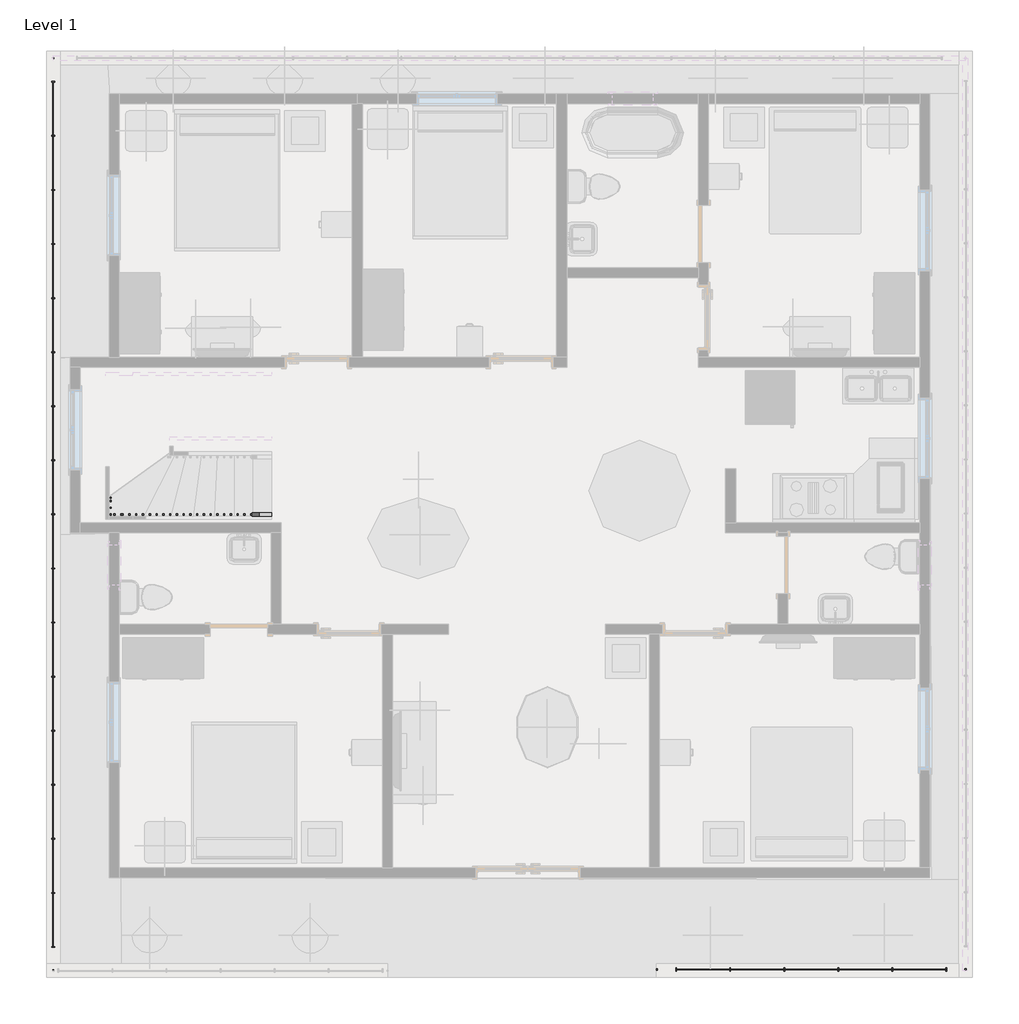
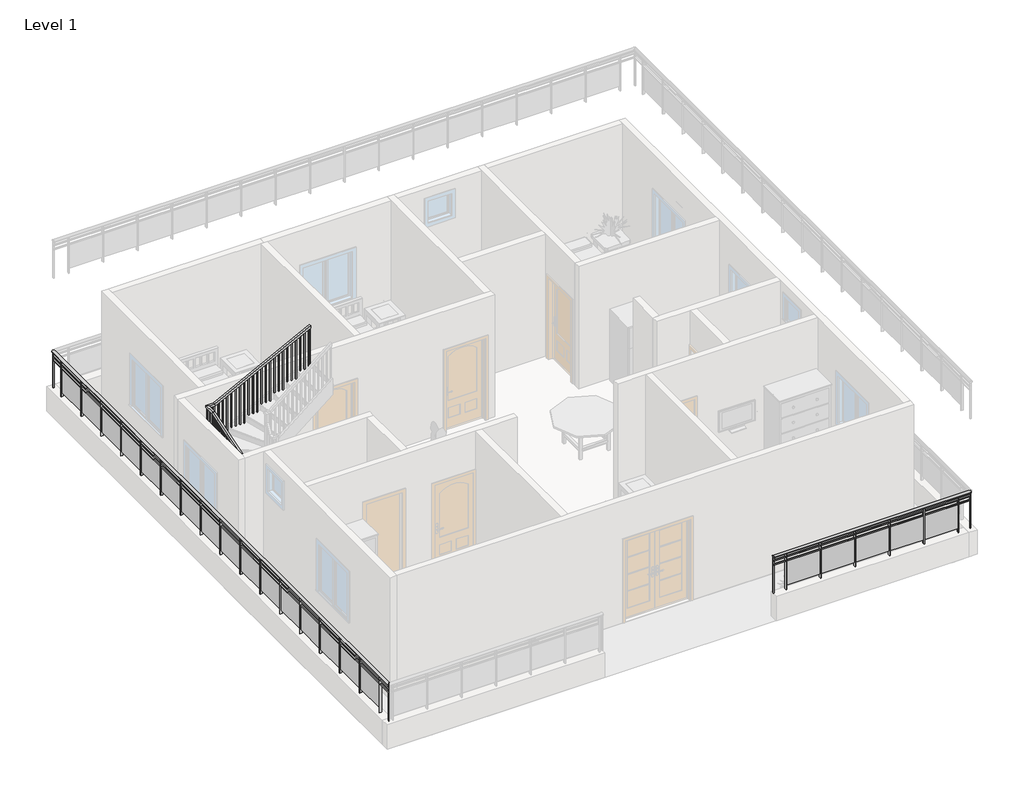
# One storey, part 2 of 5: 3 railings.
"""IFC4 building model written with IfcOpenShell, lengths in millimetres."""

from ifc_helpers import new_model, si_unit, point, frame, origin, place, context, project, spatial, polyline, ellipse_curve, trimmed, outline, extrude, faceted_brep, element, save
from ifc_brep_helpers import plane_surface, extruded_surface, advanced_brep

model = new_model("IFC4")

# Units and contexts
model_context = context("Model", 3, world=origin())
ifc_project = project(units=[si_unit("LENGTHUNIT", "METRE", prefix="MILLI")], contexts=[model_context])

# Site, building, storey
site = spatial("IfcSite", under=ifc_project)
building = spatial("IfcBuilding", under=site)
storey = spatial("IfcBuildingStorey", under=building, Name="Level 1", Elevation=0.0)

# Railings
placement = place(None, origin())
element("IfcRailing", 1, ObjectType="Glass Panel - Bottom Fill", at=placement, inside=storey, context=model_context, shape_type="SolidModel", body=[
    advanced_brep(
    [(2243.3065334, 607.1216937, 1524.0), (2243.3065334, 683.3216937, 1524.0), (-2404.8934666, 607.1216937, 1524.0), (-2404.8934666, 683.3216937, 1524.0)],
    [
        (0, 1, ellipse_curve(frame((2243.3065334, 645.2216937, 1524.0), z_axis=(1.0, 0.0, 0.0), x_axis=(0.0, 1.0, 0.0)), 38.1, 28.575)),
        (1, 0, ellipse_curve(frame((2243.3065334, 645.2216937, 1524.0), z_axis=(1.0, 0.0, 0.0), x_axis=(0.0, 1.0, 0.0)), 38.1, 28.575)),
        (2, 3, ellipse_curve(frame((-2404.8934666, 645.2216937, 1524.0), z_axis=(-1.0, 0.0, 0.0), x_axis=(0.0, 1.0, 0.0)), 38.1, 28.575)),
        (3, 2, ellipse_curve(frame((-2404.8934666, 645.2216937, 1524.0), z_axis=(-1.0, 0.0, 0.0), x_axis=(0.0, 1.0, 0.0)), 38.1, 28.575)),
        (0, 2),
        (3, 1),
    ],
    [
        plane_surface(frame((2243.3065334, 645.2216937, 1524.0), z_axis=(1.0, 0.0, 0.0), x_axis=(0.0, -1.0, 0.0))),
        plane_surface(frame((-2404.8934666, 645.2216937, 1524.0), z_axis=(-1.0, 0.0, 0.0), x_axis=(0.0, -1.0, 0.0))),
        extruded_surface(trimmed(ellipse_curve(frame((-2404.8934666, 645.2216937, 1524.0), z_axis=(1.0, 0.0, 0.0), x_axis=(0.0, 1.0, 0.0)), 38.1, 28.575), [point((-2404.8934666, 607.1216937, 1524.0))], [point((-2404.8934666, 683.3216937, 1524.0))], True, "CARTESIAN"), (4648.2, 0.0, 0.0), 4648.2),
        extruded_surface(trimmed(ellipse_curve(frame((-2404.8934666, 645.2216937, 1524.0), z_axis=(1.0, 0.0, 0.0), x_axis=(0.0, 1.0, 0.0)), 38.1, 28.575), [point((-2404.8934666, 683.3216937, 1524.0))], [point((-2404.8934666, 607.1216937, 1524.0))], True, "CARTESIAN"), (4648.2, 0.0, 0.0), 4648.2),
    ],
    [
        (0, [[1, 2]]),
        (1, [[3, 4]]),
        (2, [[-1, 5, -4, 6]]),
        (3, [[-2, -6, -3, -5]]),
    ],
),
    extrude(outline(polyline([(2243.3065334, 657.9216937), (2243.3065334, 632.5216937), (-2404.8934666, 632.5216937), (-2404.8934666, 657.9216937), (2243.3065334, 657.9216937)])), frame((0.0, 0.0, 1409.7), z_axis=(0.0, 0.0, 1.0), x_axis=(1.0, 0.0, 0.0)), (0.0, 0.0, 1.0), 25.4),
    extrude(outline(polyline([(2243.3065334, 657.9216937), (2243.3065334, 632.5216937), (-2404.8934666, 632.5216937), (-2404.8934666, 657.9216937), (2243.3065334, 657.9216937)])), frame((0.0, 0.0, 1308.1), z_axis=(0.0, 0.0, 1.0), x_axis=(1.0, 0.0, 0.0)), (0.0, 0.0, 1.0), 25.4),
    extrude(outline(polyline([(-2106.4434666, 670.6216937), (-2106.4434666, 619.8216937), (-2119.1434666, 619.8216937), (-2119.1434666, 670.6216937), (-2106.4434666, 670.6216937)])), frame((0.0, 0.0, 609.6), z_axis=(0.0, 0.0, 1.0), x_axis=(1.0, 0.0, 0.0)), (0.0, 0.0, 1.0), 885.6788223),
    extrude(outline(polyline([(-1299.9934666, 638.6865367), (-2112.7934666, 638.6865367), (-2112.7934666, 645.0365367), (-1299.9934666, 645.0365367), (-1299.9934666, 638.6865367)])), frame((0.0, 0.0, 711.2), z_axis=(0.0, 0.0, 1.0), x_axis=(1.0, 0.0, 0.0)), (0.0, 0.0, 1.0), 596.9),
    extrude(outline(polyline([(-1293.6434666, 670.6216937), (-1293.6434666, 619.8216937), (-1306.3434666, 619.8216937), (-1306.3434666, 670.6216937), (-1293.6434666, 670.6216937)])), frame((0.0, 0.0, 609.6), z_axis=(0.0, 0.0, 1.0), x_axis=(1.0, 0.0, 0.0)), (0.0, 0.0, 1.0), 885.6788223),
    extrude(outline(polyline([(-487.1934666, 638.6865367), (-1299.9934666, 638.6865367), (-1299.9934666, 645.0365367), (-487.1934666, 645.0365367), (-487.1934666, 638.6865367)])), frame((0.0, 0.0, 711.2), z_axis=(0.0, 0.0, 1.0), x_axis=(1.0, 0.0, 0.0)), (0.0, 0.0, 1.0), 596.9),
    extrude(outline(polyline([(-480.8434666, 670.6216937), (-480.8434666, 619.8216937), (-493.5434666, 619.8216937), (-493.5434666, 670.6216937), (-480.8434666, 670.6216937)])), frame((0.0, 0.0, 609.6), z_axis=(0.0, 0.0, 1.0), x_axis=(1.0, 0.0, 0.0)), (0.0, 0.0, 1.0), 885.6788223),
    extrude(outline(polyline([(325.6065334, 638.6865367), (-487.1934666, 638.6865367), (-487.1934666, 645.0365367), (325.6065334, 645.0365367), (325.6065334, 638.6865367)])), frame((0.0, 0.0, 711.2), z_axis=(0.0, 0.0, 1.0), x_axis=(1.0, 0.0, 0.0)), (0.0, 0.0, 1.0), 596.9),
    extrude(outline(polyline([(331.9565334, 670.6216937), (331.9565334, 619.8216937), (319.2565334, 619.8216937), (319.2565334, 670.6216937), (331.9565334, 670.6216937)])), frame((0.0, 0.0, 609.6), z_axis=(0.0, 0.0, 1.0), x_axis=(1.0, 0.0, 0.0)), (0.0, 0.0, 1.0), 885.6788223),
    extrude(outline(polyline([(1138.4065334, 638.6865367), (325.6065334, 638.6865367), (325.6065334, 645.0365367), (1138.4065334, 645.0365367), (1138.4065334, 638.6865367)])), frame((0.0, 0.0, 711.2), z_axis=(0.0, 0.0, 1.0), x_axis=(1.0, 0.0, 0.0)), (0.0, 0.0, 1.0), 596.9),
    extrude(outline(polyline([(1144.7565334, 670.6216937), (1144.7565334, 619.8216937), (1132.0565334, 619.8216937), (1132.0565334, 670.6216937), (1144.7565334, 670.6216937)])), frame((0.0, 0.0, 609.6), z_axis=(0.0, 0.0, 1.0), x_axis=(1.0, 0.0, 0.0)), (0.0, 0.0, 1.0), 885.6788223),
    extrude(outline(polyline([(1951.2065334, 638.6865367), (1138.4065334, 638.6865367), (1138.4065334, 645.0365367), (1951.2065334, 645.0365367), (1951.2065334, 638.6865367)])), frame((0.0, 0.0, 711.2), z_axis=(0.0, 0.0, 1.0), x_axis=(1.0, 0.0, 0.0)), (0.0, 0.0, 1.0), 596.9),
    extrude(outline(polyline([(1957.5565334, 670.6216937), (1957.5565334, 619.8216937), (1944.8565334, 619.8216937), (1944.8565334, 670.6216937), (1957.5565334, 670.6216937)])), frame((0.0, 0.0, 609.6), z_axis=(0.0, 0.0, 1.0), x_axis=(1.0, 0.0, 0.0)), (0.0, 0.0, 1.0), 885.6788223),
    extrude(outline(polyline([(-2392.1934666, 654.7466937), (-2392.1934666, 635.6966937), (-2411.2434666, 635.6966937), (-2411.2434666, 654.7466937), (-2392.1934666, 654.7466937)])), frame((0.0, 0.0, 609.6), z_axis=(0.0, 0.0, 1.0), x_axis=(1.0, 0.0, 0.0)), (0.0, 0.0, 1.0), 885.6788223),
    extrude(outline(polyline([(2249.6565334, 654.7466937), (2249.6565334, 635.6966937), (2230.6065334, 635.6966937), (2230.6065334, 654.7466937), (2249.6565334, 654.7466937)])), frame((0.0, 0.0, 609.6), z_axis=(0.0, 0.0, 1.0), x_axis=(1.0, 0.0, 0.0)), (0.0, 0.0, 1.0), 885.6788223),
])
element("IfcRailing", 2, ObjectType="Glass Panel - Bottom Fill", at=placement, inside=storey, context=model_context, shape_type="SolidModel", body=[
    advanced_brep(
    [(-11517.1434666, 626.1716937, 1524.0), (-11440.9434666, 626.1716937, 1524.0), (-11517.1434666, 14342.1716937, 1524.0), (-11440.9434666, 14342.1716937, 1524.0)],
    [
        (0, 1, ellipse_curve(frame((-11479.0434666, 626.1716937, 1524.0), z_axis=(0.0, -1.0, 0.0), x_axis=(1.0, 0.0, 0.0)), 38.1, 28.575)),
        (1, 0, ellipse_curve(frame((-11479.0434666, 626.1716937, 1524.0), z_axis=(0.0, -1.0, 0.0), x_axis=(1.0, 0.0, 0.0)), 38.1, 28.575)),
        (2, 3, ellipse_curve(frame((-11479.0434666, 14342.1716937, 1524.0), z_axis=(0.0, 1.0, 0.0), x_axis=(1.0, 0.0, 0.0)), 38.1, 28.575)),
        (3, 2, ellipse_curve(frame((-11479.0434666, 14342.1716937, 1524.0), z_axis=(0.0, 1.0, 0.0), x_axis=(1.0, 0.0, 0.0)), 38.1, 28.575)),
        (0, 2),
        (3, 1),
    ],
    [
        plane_surface(frame((-11479.0434666, 626.1716937, 1524.0), z_axis=(0.0, -1.0, 0.0), x_axis=(0.0, 0.0, 1.0))),
        plane_surface(frame((-11479.0434666, 14342.1716937, 1524.0), z_axis=(0.0, 1.0, 0.0), x_axis=(0.0, 0.0, 1.0))),
        extruded_surface(trimmed(ellipse_curve(frame((-11479.0434666, 14342.1716937, 1524.0), z_axis=(0.0, -1.0, 0.0), x_axis=(1.0, 0.0, 0.0)), 38.1, 28.575), [point((-11517.1434666, 14342.1716937, 1524.0))], [point((-11440.9434666, 14342.1716937, 1524.0))], True, "CARTESIAN"), (0.0, -13716.0, 0.0), 13716.0),
        extruded_surface(trimmed(ellipse_curve(frame((-11479.0434666, 14342.1716937, 1524.0), z_axis=(0.0, -1.0, 0.0), x_axis=(1.0, 0.0, 0.0)), 38.1, 28.575), [point((-11440.9434666, 14342.1716937, 1524.0))], [point((-11517.1434666, 14342.1716937, 1524.0))], True, "CARTESIAN"), (0.0, -13716.0, 0.0), 13716.0),
    ],
    [
        (0, [[1, 2]]),
        (1, [[3, 4]]),
        (2, [[-1, 5, -4, 6]]),
        (3, [[-2, -6, -3, -5]]),
    ],
),
    extrude(outline(polyline([(-11466.3434666, 626.1716937), (-11491.7434666, 626.1716937), (-11491.7434666, 14342.1716937), (-11466.3434666, 14342.1716937), (-11466.3434666, 626.1716937)])), frame((0.0, 0.0, 1409.7), z_axis=(0.0, 0.0, 1.0), x_axis=(1.0, 0.0, 0.0)), (0.0, 0.0, 1.0), 25.4),
    extrude(outline(polyline([(-11466.3434666, 626.1716937), (-11491.7434666, 626.1716937), (-11491.7434666, 14342.1716937), (-11466.3434666, 14342.1716937), (-11466.3434666, 626.1716937)])), frame((0.0, 0.0, 1308.1), z_axis=(0.0, 0.0, 1.0), x_axis=(1.0, 0.0, 0.0)), (0.0, 0.0, 1.0), 25.4),
    extrude(outline(polyline([(-11453.6434666, 13980.2216937), (-11504.4434666, 13980.2216937), (-11504.4434666, 13992.9216937), (-11453.6434666, 13992.9216937), (-11453.6434666, 13980.2216937)])), frame((0.0, 0.0, 609.6), z_axis=(0.0, 0.0, 1.0), x_axis=(1.0, 0.0, 0.0)), (0.0, 0.0, 1.0), 885.6788223),
    extrude(outline(polyline([(-11485.5786236, 13173.7716937), (-11485.5786236, 13986.5716937), (-11479.2286236, 13986.5716937), (-11479.2286236, 13173.7716937), (-11485.5786236, 13173.7716937)])), frame((0.0, 0.0, 711.2), z_axis=(0.0, 0.0, 1.0), x_axis=(1.0, 0.0, 0.0)), (0.0, 0.0, 1.0), 596.9),
    extrude(outline(polyline([(-11453.6434666, 13167.4216937), (-11504.4434666, 13167.4216937), (-11504.4434666, 13180.1216937), (-11453.6434666, 13180.1216937), (-11453.6434666, 13167.4216937)])), frame((0.0, 0.0, 609.6), z_axis=(0.0, 0.0, 1.0), x_axis=(1.0, 0.0, 0.0)), (0.0, 0.0, 1.0), 885.6788223),
    extrude(outline(polyline([(-11485.5786236, 12360.9716937), (-11485.5786236, 13173.7716937), (-11479.2286236, 13173.7716937), (-11479.2286236, 12360.9716937), (-11485.5786236, 12360.9716937)])), frame((0.0, 0.0, 711.2), z_axis=(0.0, 0.0, 1.0), x_axis=(1.0, 0.0, 0.0)), (0.0, 0.0, 1.0), 596.9),
    extrude(outline(polyline([(-11453.6434666, 12354.6216937), (-11504.4434666, 12354.6216937), (-11504.4434666, 12367.3216937), (-11453.6434666, 12367.3216937), (-11453.6434666, 12354.6216937)])), frame((0.0, 0.0, 609.6), z_axis=(0.0, 0.0, 1.0), x_axis=(1.0, 0.0, 0.0)), (0.0, 0.0, 1.0), 885.6788223),
    extrude(outline(polyline([(-11485.5786236, 11548.1716937), (-11485.5786236, 12360.9716937), (-11479.2286236, 12360.9716937), (-11479.2286236, 11548.1716937), (-11485.5786236, 11548.1716937)])), frame((0.0, 0.0, 711.2), z_axis=(0.0, 0.0, 1.0), x_axis=(1.0, 0.0, 0.0)), (0.0, 0.0, 1.0), 596.9),
    extrude(outline(polyline([(-11453.6434666, 11541.8216937), (-11504.4434666, 11541.8216937), (-11504.4434666, 11554.5216937), (-11453.6434666, 11554.5216937), (-11453.6434666, 11541.8216937)])), frame((0.0, 0.0, 609.6), z_axis=(0.0, 0.0, 1.0), x_axis=(1.0, 0.0, 0.0)), (0.0, 0.0, 1.0), 885.6788223),
    extrude(outline(polyline([(-11485.5786236, 10735.3716937), (-11485.5786236, 11548.1716937), (-11479.2286236, 11548.1716937), (-11479.2286236, 10735.3716937), (-11485.5786236, 10735.3716937)])), frame((0.0, 0.0, 711.2), z_axis=(0.0, 0.0, 1.0), x_axis=(1.0, 0.0, 0.0)), (0.0, 0.0, 1.0), 596.9),
    extrude(outline(polyline([(-11453.6434666, 10729.0216937), (-11504.4434666, 10729.0216937), (-11504.4434666, 10741.7216937), (-11453.6434666, 10741.7216937), (-11453.6434666, 10729.0216937)])), frame((0.0, 0.0, 609.6), z_axis=(0.0, 0.0, 1.0), x_axis=(1.0, 0.0, 0.0)), (0.0, 0.0, 1.0), 885.6788223),
    extrude(outline(polyline([(-11485.5786236, 9922.5716937), (-11485.5786236, 10735.3716937), (-11479.2286236, 10735.3716937), (-11479.2286236, 9922.5716937), (-11485.5786236, 9922.5716937)])), frame((0.0, 0.0, 711.2), z_axis=(0.0, 0.0, 1.0), x_axis=(1.0, 0.0, 0.0)), (0.0, 0.0, 1.0), 596.9),
    extrude(outline(polyline([(-11453.6434666, 9916.2216937), (-11504.4434666, 9916.2216937), (-11504.4434666, 9928.9216937), (-11453.6434666, 9928.9216937), (-11453.6434666, 9916.2216937)])), frame((0.0, 0.0, 609.6), z_axis=(0.0, 0.0, 1.0), x_axis=(1.0, 0.0, 0.0)), (0.0, 0.0, 1.0), 885.6788223),
    extrude(outline(polyline([(-11485.5786236, 9109.7716937), (-11485.5786236, 9922.5716937), (-11479.2286236, 9922.5716937), (-11479.2286236, 9109.7716937), (-11485.5786236, 9109.7716937)])), frame((0.0, 0.0, 711.2), z_axis=(0.0, 0.0, 1.0), x_axis=(1.0, 0.0, 0.0)), (0.0, 0.0, 1.0), 596.9),
    extrude(outline(polyline([(-11453.6434666, 9103.4216937), (-11504.4434666, 9103.4216937), (-11504.4434666, 9116.1216937), (-11453.6434666, 9116.1216937), (-11453.6434666, 9103.4216937)])), frame((0.0, 0.0, 609.6), z_axis=(0.0, 0.0, 1.0), x_axis=(1.0, 0.0, 0.0)), (0.0, 0.0, 1.0), 885.6788223),
    extrude(outline(polyline([(-11485.5786236, 8296.9716937), (-11485.5786236, 9109.7716937), (-11479.2286236, 9109.7716937), (-11479.2286236, 8296.9716937), (-11485.5786236, 8296.9716937)])), frame((0.0, 0.0, 711.2), z_axis=(0.0, 0.0, 1.0), x_axis=(1.0, 0.0, 0.0)), (0.0, 0.0, 1.0), 596.9),
    extrude(outline(polyline([(-11453.6434666, 8290.6216937), (-11504.4434666, 8290.6216937), (-11504.4434666, 8303.3216937), (-11453.6434666, 8303.3216937), (-11453.6434666, 8290.6216937)])), frame((0.0, 0.0, 609.6), z_axis=(0.0, 0.0, 1.0), x_axis=(1.0, 0.0, 0.0)), (0.0, 0.0, 1.0), 885.6788223),
    extrude(outline(polyline([(-11485.5786236, 7484.1716937), (-11485.5786236, 8296.9716937), (-11479.2286236, 8296.9716937), (-11479.2286236, 7484.1716937), (-11485.5786236, 7484.1716937)])), frame((0.0, 0.0, 711.2), z_axis=(0.0, 0.0, 1.0), x_axis=(1.0, 0.0, 0.0)), (0.0, 0.0, 1.0), 596.9),
    extrude(outline(polyline([(-11453.6434666, 7477.8216937), (-11504.4434666, 7477.8216937), (-11504.4434666, 7490.5216937), (-11453.6434666, 7490.5216937), (-11453.6434666, 7477.8216937)])), frame((0.0, 0.0, 609.6), z_axis=(0.0, 0.0, 1.0), x_axis=(1.0, 0.0, 0.0)), (0.0, 0.0, 1.0), 885.6788223),
    extrude(outline(polyline([(-11485.5786236, 6671.3716937), (-11485.5786236, 7484.1716937), (-11479.2286236, 7484.1716937), (-11479.2286236, 6671.3716937), (-11485.5786236, 6671.3716937)])), frame((0.0, 0.0, 711.2), z_axis=(0.0, 0.0, 1.0), x_axis=(1.0, 0.0, 0.0)), (0.0, 0.0, 1.0), 596.9),
    extrude(outline(polyline([(-11453.6434666, 6665.0216937), (-11504.4434666, 6665.0216937), (-11504.4434666, 6677.7216937), (-11453.6434666, 6677.7216937), (-11453.6434666, 6665.0216937)])), frame((0.0, 0.0, 609.6), z_axis=(0.0, 0.0, 1.0), x_axis=(1.0, 0.0, 0.0)), (0.0, 0.0, 1.0), 885.6788223),
    extrude(outline(polyline([(-11485.5786236, 5858.5716937), (-11485.5786236, 6671.3716937), (-11479.2286236, 6671.3716937), (-11479.2286236, 5858.5716937), (-11485.5786236, 5858.5716937)])), frame((0.0, 0.0, 711.2), z_axis=(0.0, 0.0, 1.0), x_axis=(1.0, 0.0, 0.0)), (0.0, 0.0, 1.0), 596.9),
    extrude(outline(polyline([(-11453.6434666, 5852.2216937), (-11504.4434666, 5852.2216937), (-11504.4434666, 5864.9216937), (-11453.6434666, 5864.9216937), (-11453.6434666, 5852.2216937)])), frame((0.0, 0.0, 609.6), z_axis=(0.0, 0.0, 1.0), x_axis=(1.0, 0.0, 0.0)), (0.0, 0.0, 1.0), 885.6788223),
    extrude(outline(polyline([(-11485.5786236, 5045.7716937), (-11485.5786236, 5858.5716937), (-11479.2286236, 5858.5716937), (-11479.2286236, 5045.7716937), (-11485.5786236, 5045.7716937)])), frame((0.0, 0.0, 711.2), z_axis=(0.0, 0.0, 1.0), x_axis=(1.0, 0.0, 0.0)), (0.0, 0.0, 1.0), 596.9),
    extrude(outline(polyline([(-11453.6434666, 5039.4216937), (-11504.4434666, 5039.4216937), (-11504.4434666, 5052.1216937), (-11453.6434666, 5052.1216937), (-11453.6434666, 5039.4216937)])), frame((0.0, 0.0, 609.6), z_axis=(0.0, 0.0, 1.0), x_axis=(1.0, 0.0, 0.0)), (0.0, 0.0, 1.0), 885.6788223),
    extrude(outline(polyline([(-11485.5786236, 4232.9716937), (-11485.5786236, 5045.7716937), (-11479.2286236, 5045.7716937), (-11479.2286236, 4232.9716937), (-11485.5786236, 4232.9716937)])), frame((0.0, 0.0, 711.2), z_axis=(0.0, 0.0, 1.0), x_axis=(1.0, 0.0, 0.0)), (0.0, 0.0, 1.0), 596.9),
    extrude(outline(polyline([(-11453.6434666, 4226.6216937), (-11504.4434666, 4226.6216937), (-11504.4434666, 4239.3216937), (-11453.6434666, 4239.3216937), (-11453.6434666, 4226.6216937)])), frame((0.0, 0.0, 609.6), z_axis=(0.0, 0.0, 1.0), x_axis=(1.0, 0.0, 0.0)), (0.0, 0.0, 1.0), 885.6788223),
    extrude(outline(polyline([(-11485.5786236, 3420.1716937), (-11485.5786236, 4232.9716937), (-11479.2286236, 4232.9716937), (-11479.2286236, 3420.1716937), (-11485.5786236, 3420.1716937)])), frame((0.0, 0.0, 711.2), z_axis=(0.0, 0.0, 1.0), x_axis=(1.0, 0.0, 0.0)), (0.0, 0.0, 1.0), 596.9),
    extrude(outline(polyline([(-11453.6434666, 3413.8216937), (-11504.4434666, 3413.8216937), (-11504.4434666, 3426.5216937), (-11453.6434666, 3426.5216937), (-11453.6434666, 3413.8216937)])), frame((0.0, 0.0, 609.6), z_axis=(0.0, 0.0, 1.0), x_axis=(1.0, 0.0, 0.0)), (0.0, 0.0, 1.0), 885.6788223),
    extrude(outline(polyline([(-11485.5786236, 2607.3716937), (-11485.5786236, 3420.1716937), (-11479.2286236, 3420.1716937), (-11479.2286236, 2607.3716937), (-11485.5786236, 2607.3716937)])), frame((0.0, 0.0, 711.2), z_axis=(0.0, 0.0, 1.0), x_axis=(1.0, 0.0, 0.0)), (0.0, 0.0, 1.0), 596.9),
    extrude(outline(polyline([(-11453.6434666, 2601.0216937), (-11504.4434666, 2601.0216937), (-11504.4434666, 2613.7216937), (-11453.6434666, 2613.7216937), (-11453.6434666, 2601.0216937)])), frame((0.0, 0.0, 609.6), z_axis=(0.0, 0.0, 1.0), x_axis=(1.0, 0.0, 0.0)), (0.0, 0.0, 1.0), 885.6788223),
    extrude(outline(polyline([(-11485.5786236, 1794.5716937), (-11485.5786236, 2607.3716937), (-11479.2286236, 2607.3716937), (-11479.2286236, 1794.5716937), (-11485.5786236, 1794.5716937)])), frame((0.0, 0.0, 711.2), z_axis=(0.0, 0.0, 1.0), x_axis=(1.0, 0.0, 0.0)), (0.0, 0.0, 1.0), 596.9),
    extrude(outline(polyline([(-11453.6434666, 1788.2216937), (-11504.4434666, 1788.2216937), (-11504.4434666, 1800.9216937), (-11453.6434666, 1800.9216937), (-11453.6434666, 1788.2216937)])), frame((0.0, 0.0, 609.6), z_axis=(0.0, 0.0, 1.0), x_axis=(1.0, 0.0, 0.0)), (0.0, 0.0, 1.0), 885.6788223),
    extrude(outline(polyline([(-11485.5786236, 981.7716937), (-11485.5786236, 1794.5716937), (-11479.2286236, 1794.5716937), (-11479.2286236, 981.7716937), (-11485.5786236, 981.7716937)])), frame((0.0, 0.0, 711.2), z_axis=(0.0, 0.0, 1.0), x_axis=(1.0, 0.0, 0.0)), (0.0, 0.0, 1.0), 596.9),
    extrude(outline(polyline([(-11453.6434666, 975.4216937), (-11504.4434666, 975.4216937), (-11504.4434666, 988.1216937), (-11453.6434666, 988.1216937), (-11453.6434666, 975.4216937)])), frame((0.0, 0.0, 609.6), z_axis=(0.0, 0.0, 1.0), x_axis=(1.0, 0.0, 0.0)), (0.0, 0.0, 1.0), 885.6788223),
    extrude(outline(polyline([(-11469.5184666, 14329.4716937), (-11488.5684666, 14329.4716937), (-11488.5684666, 14348.5216937), (-11469.5184666, 14348.5216937), (-11469.5184666, 14329.4716937)])), frame((0.0, 0.0, 609.6), z_axis=(0.0, 0.0, 1.0), x_axis=(1.0, 0.0, 0.0)), (0.0, 0.0, 1.0), 885.6788223),
    extrude(outline(polyline([(-11469.5184666, 619.8216937), (-11488.5684666, 619.8216937), (-11488.5684666, 638.8716937), (-11469.5184666, 638.8716937), (-11469.5184666, 619.8216937)])), frame((0.0, 0.0, 609.6), z_axis=(0.0, 0.0, 1.0), x_axis=(1.0, 0.0, 0.0)), (0.0, 0.0, 1.0), 885.6788223),
])
element("IfcRailing", 3, ObjectType="Handrail - Rectangular", at=placement, inside=storey, context=model_context, shape_type="SolidModel", body=[
    faceted_brep([(-8198.7117747, 7458.7716937, 1109.0771751), (-8198.7117747, 7458.7716937, 1051.9280057), (-8198.7117747, 7509.5716937, 1051.9280057), (-8198.7117747, 7509.5716937, 1109.0771751), (-10458.6936312, 7458.7716937, 2273.7644996), (-10471.0136825, 7458.7716937, 2222.9644996), (-10471.0136825, 7509.5716937, 2222.9644996), (-10458.6936312, 7509.5716937, 2273.7644996), (-10640.8434666, 7458.7716937, 2273.7644996), (-10640.8434666, 7458.7716937, 2222.9644996), (-10590.0434666, 7509.5716937, 2222.9644996), (-10590.0434666, 7509.5716937, 2273.7644996), (-10640.8434666, 7735.9256463, 2273.7644996), (-10640.8434666, 7743.8762225, 2222.9644996), (-10590.0434666, 7743.8762225, 2222.9644996), (-10590.0434666, 7735.9256463, 2273.7644996), (-10640.8434666, 9289.8177411, 2772.3688337), (-10640.8434666, 9297.7683172, 2721.5688337), (-10590.0434666, 9297.7683172, 2721.5688337), (-10590.0434666, 9289.8177411, 2772.3688337), (-10640.8434666, 9566.9716937, 2772.3688337), (-10640.8434666, 9566.9716937, 2721.5688337), (-10590.0434666, 9516.1716937, 2721.5688337), (-10590.0434666, 9516.1716937, 2772.3688337), (-10458.6936312, 9566.9716937, 2772.3688337), (-10446.3735799, 9566.9716937, 2721.5688337), (-10446.3735799, 9516.1716937, 2721.5688337), (-10458.6936312, 9516.1716937, 2772.3688337), (-8198.7117747, 9566.9716937, 3937.0561582), (-8198.7117747, 9516.1716937, 3937.0561582), (-8198.7117747, 9516.1716937, 3879.9069889), (-8198.7117747, 9566.9716937, 3879.9069889)], [[[0, 1, 2, 3]], [[1, 0, 4, 5]], [[2, 1, 5, 6]], [[3, 2, 6, 7]], [[0, 3, 7, 4]], [[5, 4, 8, 9]], [[6, 5, 9, 10]], [[7, 6, 10, 11]], [[4, 7, 11, 8]], [[9, 8, 12, 13]], [[10, 9, 13, 14]], [[11, 10, 14, 15]], [[8, 11, 15, 12]], [[13, 12, 16, 17]], [[14, 13, 17, 18]], [[15, 14, 18, 19]], [[12, 15, 19, 16]], [[17, 16, 20, 21]], [[18, 17, 21, 22]], [[19, 18, 22, 23]], [[16, 19, 23, 20]], [[21, 20, 24, 25]], [[22, 21, 25, 26]], [[23, 22, 26, 27]], [[20, 23, 27, 24]], [[28, 29, 30, 31]], [[25, 24, 28, 31]], [[26, 25, 31, 30]], [[27, 26, 30, 29]], [[24, 27, 29, 28]]]),
    extrude(outline(polyline([(3862.2268642, -8233.0186312), (2878.6666667, -8233.0186312), (2878.6666667, -8213.9686312), (3872.0443296, -8213.9686312), (3862.2268642, -8233.0186312)])), frame((0.0, 9532.0466937, 0.0), z_axis=(0.0, 1.0, 0.0), x_axis=(0.0, 0.0, 1.0)), (0.0, 0.0, 1.0), 19.05),
    extrude(outline(polyline([(3809.8670491, -8334.6186312), (2878.6666667, -8334.6186312), (2878.6666667, -8315.5686312), (3819.6845145, -8315.5686312), (3809.8670491, -8334.6186312)])), frame((0.0, 9532.0466937, 0.0), z_axis=(0.0, 1.0, 0.0), x_axis=(0.0, 0.0, 1.0)), (0.0, 0.0, 1.0), 19.05),
    extrude(outline(polyline([(3757.507234, -8436.2186312), (2878.6666667, -8436.2186312), (2878.6666667, -8417.1686312), (3767.3246993, -8417.1686312), (3757.507234, -8436.2186312)])), frame((0.0, 9532.0466937, 0.0), z_axis=(0.0, 1.0, 0.0), x_axis=(0.0, 0.0, 1.0)), (0.0, 0.0, 1.0), 19.05),
    extrude(outline(polyline([(3705.1474189, -8537.8186312), (2709.3333333, -8537.8186312), (2709.3333333, -8518.7686312), (3714.9648842, -8518.7686312), (3705.1474189, -8537.8186312)])), frame((0.0, 9532.0466937, 0.0), z_axis=(0.0, 1.0, 0.0), x_axis=(0.0, 0.0, 1.0)), (0.0, 0.0, 1.0), 19.05),
    extrude(outline(polyline([(3652.7876038, -8639.4186312), (2709.3333333, -8639.4186312), (2709.3333333, -8620.3686312), (3662.6050691, -8620.3686312), (3652.7876038, -8639.4186312)])), frame((0.0, 9532.0466937, 0.0), z_axis=(0.0, 1.0, 0.0), x_axis=(0.0, 0.0, 1.0)), (0.0, 0.0, 1.0), 19.05),
    extrude(outline(polyline([(3600.4277887, -8741.0186312), (2709.3333333, -8741.0186312), (2709.3333333, -8721.9686312), (3610.245254, -8721.9686312), (3600.4277887, -8741.0186312)])), frame((0.0, 9532.0466937, 0.0), z_axis=(0.0, 1.0, 0.0), x_axis=(0.0, 0.0, 1.0)), (0.0, 0.0, 1.0), 19.05),
    extrude(outline(polyline([(3548.0679735, -8842.6186312), (2540.0, -8842.6186312), (2540.0, -8823.5686312), (3557.8854389, -8823.5686312), (3548.0679735, -8842.6186312)])), frame((0.0, 9532.0466937, 0.0), z_axis=(0.0, 1.0, 0.0), x_axis=(0.0, 0.0, 1.0)), (0.0, 0.0, 1.0), 19.05),
    extrude(outline(polyline([(3495.7081584, -8944.2186312), (2540.0, -8944.2186312), (2540.0, -8925.1686312), (3505.5256238, -8925.1686312), (3495.7081584, -8944.2186312)])), frame((0.0, 9532.0466937, 0.0), z_axis=(0.0, 1.0, 0.0), x_axis=(0.0, 0.0, 1.0)), (0.0, 0.0, 1.0), 19.05),
    extrude(outline(polyline([(3443.3483433, -9045.8186312), (2540.0, -9045.8186312), (2540.0, -9026.7686312), (3453.1658086, -9026.7686312), (3443.3483433, -9045.8186312)])), frame((0.0, 9532.0466937, 0.0), z_axis=(0.0, 1.0, 0.0), x_axis=(0.0, 0.0, 1.0)), (0.0, 0.0, 1.0), 19.05),
    extrude(outline(polyline([(3390.9885282, -9147.4186312), (2370.6666667, -9147.4186312), (2370.6666667, -9128.3686312), (3400.8059935, -9128.3686312), (3390.9885282, -9147.4186312)])), frame((0.0, 9532.0466937, 0.0), z_axis=(0.0, 1.0, 0.0), x_axis=(0.0, 0.0, 1.0)), (0.0, 0.0, 1.0), 19.05),
    extrude(outline(polyline([(3338.6287131, -9249.0186312), (2370.6666667, -9249.0186312), (2370.6666667, -9229.9686312), (3348.4461784, -9229.9686312), (3338.6287131, -9249.0186312)])), frame((0.0, 9532.0466937, 0.0), z_axis=(0.0, 1.0, 0.0), x_axis=(0.0, 0.0, 1.0)), (0.0, 0.0, 1.0), 19.05),
    extrude(outline(polyline([(3286.268898, -9350.6186312), (2370.6666667, -9350.6186312), (2370.6666667, -9331.5686312), (3296.0863633, -9331.5686312), (3286.268898, -9350.6186312)])), frame((0.0, 9532.0466937, 0.0), z_axis=(0.0, 1.0, 0.0), x_axis=(0.0, 0.0, 1.0)), (0.0, 0.0, 1.0), 19.05),
    extrude(outline(polyline([(3233.9090828, -9452.2186312), (2201.3333333, -9452.2186312), (2201.3333333, -9433.1686312), (3243.7265482, -9433.1686312), (3233.9090828, -9452.2186312)])), frame((0.0, 9532.0466937, 0.0), z_axis=(0.0, 1.0, 0.0), x_axis=(0.0, 0.0, 1.0)), (0.0, 0.0, 1.0), 19.05),
    extrude(outline(polyline([(3181.5492677, -9553.8186312), (2201.3333333, -9553.8186312), (2201.3333333, -9534.7686312), (3191.3667331, -9534.7686312), (3181.5492677, -9553.8186312)])), frame((0.0, 9532.0466937, 0.0), z_axis=(0.0, 1.0, 0.0), x_axis=(0.0, 0.0, 1.0)), (0.0, 0.0, 1.0), 19.05),
    extrude(outline(polyline([(3129.1894526, -9655.4186312), (2201.3333333, -9655.4186312), (2201.3333333, -9636.3686312), (3139.0069179, -9636.3686312), (3129.1894526, -9655.4186312)])), frame((0.0, 9532.0466937, 0.0), z_axis=(0.0, 1.0, 0.0), x_axis=(0.0, 0.0, 1.0)), (0.0, 0.0, 1.0), 19.05),
    extrude(outline(polyline([(3076.8296375, -9757.0186312), (2032.0, -9757.0186312), (2032.0, -9737.9686312), (3086.6471028, -9737.9686312), (3076.8296375, -9757.0186312)])), frame((0.0, 9532.0466937, 0.0), z_axis=(0.0, 1.0, 0.0), x_axis=(0.0, 0.0, 1.0)), (0.0, 0.0, 1.0), 19.05),
    extrude(outline(polyline([(3024.4698224, -9858.6186312), (2032.0, -9858.6186312), (2032.0, -9839.5686312), (3034.2872877, -9839.5686312), (3024.4698224, -9858.6186312)])), frame((0.0, 9532.0466937, 0.0), z_axis=(0.0, 1.0, 0.0), x_axis=(0.0, 0.0, 1.0)), (0.0, 0.0, 1.0), 19.05),
    extrude(outline(polyline([(2972.1100073, -9960.2186312), (2032.0, -9960.2186312), (2032.0, -9941.1686312), (2981.9274726, -9941.1686312), (2972.1100073, -9960.2186312)])), frame((0.0, 9532.0466937, 0.0), z_axis=(0.0, 1.0, 0.0), x_axis=(0.0, 0.0, 1.0)), (0.0, 0.0, 1.0), 19.05),
    extrude(outline(polyline([(2919.7501921, -10061.8186312), (2032.0, -10061.8186312), (2032.0, -10042.7686312), (2929.5676575, -10042.7686312), (2919.7501921, -10061.8186312)])), frame((0.0, 9532.0466937, 0.0), z_axis=(0.0, 1.0, 0.0), x_axis=(0.0, 0.0, 1.0)), (0.0, 0.0, 1.0), 19.05),
    extrude(outline(polyline([(2867.390377, -10163.4186312), (1862.6666667, -10163.4186312), (1862.6666667, -10144.3686312), (2877.2078424, -10144.3686312), (2867.390377, -10163.4186312)])), frame((0.0, 9532.0466937, 0.0), z_axis=(0.0, 1.0, 0.0), x_axis=(0.0, 0.0, 1.0)), (0.0, 0.0, 1.0), 19.05),
    extrude(outline(polyline([(2815.0305619, -10265.0186312), (1862.6666667, -10265.0186312), (1862.6666667, -10245.9686312), (2824.8480272, -10245.9686312), (2815.0305619, -10265.0186312)])), frame((0.0, 9532.0466937, 0.0), z_axis=(0.0, 1.0, 0.0), x_axis=(0.0, 0.0, 1.0)), (0.0, 0.0, 1.0), 19.05),
    extrude(outline(polyline([(2762.6707468, -10366.6186312), (1862.6666667, -10366.6186312), (1862.6666667, -10347.5686312), (2772.4882121, -10347.5686312), (2762.6707468, -10366.6186312)])), frame((0.0, 9532.0466937, 0.0), z_axis=(0.0, 1.0, 0.0), x_axis=(0.0, 0.0, 1.0)), (0.0, 0.0, 1.0), 19.05),
    extrude(outline(polyline([(-10523.3684666, 9551.0966937), (-10504.3184666, 9551.0966937), (-10504.3184666, 9532.0466937), (-10523.3684666, 9532.0466937), (-10523.3684666, 9551.0966937)])), frame((0.0, 0.0, 1862.6666667), z_axis=(0.0, 0.0, 1.0), x_axis=(1.0, 0.0, 0.0)), (0.0, 0.0, 1.0), 858.902167),
    extrude(outline(polyline([(-10624.9684666, 9483.4927411), (-10624.9684666, 9502.5427411), (-10605.9184666, 9502.5427411), (-10605.9184666, 9483.4927411), (-10624.9684666, 9483.4927411)])), frame((0.0, 0.0, 1862.6666667), z_axis=(0.0, 0.0, 1.0), x_axis=(1.0, 0.0, 0.0)), (0.0, 0.0, 1.0), 858.902167),
    extrude(outline(polyline([(-10624.9684666, 9381.8927411), (-10624.9684666, 9400.9427411), (-10605.9184666, 9400.9427411), (-10605.9184666, 9381.8927411), (-10624.9684666, 9381.8927411)])), frame((0.0, 0.0, 1862.6666667), z_axis=(0.0, 0.0, 1.0), x_axis=(1.0, 0.0, 0.0)), (0.0, 0.0, 1.0), 858.902167),
    extrude(outline(polyline([(9269.4506463, 2712.4824155), (9269.4506463, 1693.3333333), (9250.4006463, 1693.3333333), (9250.4006463, 2706.3697564), (9269.4506463, 2712.4824155)])), frame((-10624.9684666, 0.0, 0.0), z_axis=(1.0, 0.0, 0.0), x_axis=(0.0, 1.0, 0.0)), (0.0, 0.0, 1.0), 19.05),
    extrude(outline(polyline([(9167.8506463, 2679.8815673), (9167.8506463, 1693.3333333), (9148.8006463, 1693.3333333), (9148.8006463, 2673.7689082), (9167.8506463, 2679.8815673)])), frame((-10624.9684666, 0.0, 0.0), z_axis=(1.0, 0.0, 0.0), x_axis=(0.0, 1.0, 0.0)), (0.0, 0.0, 1.0), 19.05),
    extrude(outline(polyline([(9066.2506463, 2647.280719), (9066.2506463, 1693.3333333), (9047.2006463, 1693.3333333), (9047.2006463, 2641.16806), (9066.2506463, 2647.280719)])), frame((-10624.9684666, 0.0, 0.0), z_axis=(1.0, 0.0, 0.0), x_axis=(0.0, 1.0, 0.0)), (0.0, 0.0, 1.0), 19.05),
    extrude(outline(polyline([(8964.6506463, 2614.6798708), (8964.6506463, 1693.3333333), (8945.6006463, 1693.3333333), (8945.6006463, 2608.5672118), (8964.6506463, 2614.6798708)])), frame((-10624.9684666, 0.0, 0.0), z_axis=(1.0, 0.0, 0.0), x_axis=(0.0, 1.0, 0.0)), (0.0, 0.0, 1.0), 19.05),
    extrude(outline(polyline([(8863.0506463, 2582.0790226), (8863.0506463, 1693.3333333), (8844.0006463, 1693.3333333), (8844.0006463, 2575.9663635), (8863.0506463, 2582.0790226)])), frame((-10624.9684666, 0.0, 0.0), z_axis=(1.0, 0.0, 0.0), x_axis=(0.0, 1.0, 0.0)), (0.0, 0.0, 1.0), 19.05),
    extrude(outline(polyline([(8761.4506463, 2549.4781744), (8761.4506463, 1693.3333333), (8742.4006463, 1693.3333333), (8742.4006463, 2543.3655153), (8761.4506463, 2549.4781744)])), frame((-10624.9684666, 0.0, 0.0), z_axis=(1.0, 0.0, 0.0), x_axis=(0.0, 1.0, 0.0)), (0.0, 0.0, 1.0), 19.05),
    extrude(outline(polyline([(8659.8506463, 2516.8773261), (8659.8506463, 1524.0), (8640.8006463, 1524.0), (8640.8006463, 2510.7646671), (8659.8506463, 2516.8773261)])), frame((-10624.9684666, 0.0, 0.0), z_axis=(1.0, 0.0, 0.0), x_axis=(0.0, 1.0, 0.0)), (0.0, 0.0, 1.0), 19.05),
    extrude(outline(polyline([(8558.2506463, 2484.2764779), (8558.2506463, 1524.0), (8539.2006463, 1524.0), (8539.2006463, 2478.1638189), (8558.2506463, 2484.2764779)])), frame((-10624.9684666, 0.0, 0.0), z_axis=(1.0, 0.0, 0.0), x_axis=(0.0, 1.0, 0.0)), (0.0, 0.0, 1.0), 19.05),
    extrude(outline(polyline([(8456.6506463, 2451.6756297), (8456.6506463, 1524.0), (8437.6006463, 1524.0), (8437.6006463, 2445.5629706), (8456.6506463, 2451.6756297)])), frame((-10624.9684666, 0.0, 0.0), z_axis=(1.0, 0.0, 0.0), x_axis=(0.0, 1.0, 0.0)), (0.0, 0.0, 1.0), 19.05),
    extrude(outline(polyline([(8355.0506463, 2419.0747814), (8355.0506463, 1524.0), (8336.0006463, 1524.0), (8336.0006463, 2412.9621224), (8355.0506463, 2419.0747814)])), frame((-10624.9684666, 0.0, 0.0), z_axis=(1.0, 0.0, 0.0), x_axis=(0.0, 1.0, 0.0)), (0.0, 0.0, 1.0), 19.05),
    extrude(outline(polyline([(8253.4506463, 2386.4739332), (8253.4506463, 1354.6666667), (8234.4006463, 1354.6666667), (8234.4006463, 2380.3612742), (8253.4506463, 2386.4739332)])), frame((-10624.9684666, 0.0, 0.0), z_axis=(1.0, 0.0, 0.0), x_axis=(0.0, 1.0, 0.0)), (0.0, 0.0, 1.0), 19.05),
    extrude(outline(polyline([(8151.8506463, 2353.873085), (8151.8506463, 1354.6666667), (8132.8006463, 1354.6666667), (8132.8006463, 2347.7604259), (8151.8506463, 2353.873085)])), frame((-10624.9684666, 0.0, 0.0), z_axis=(1.0, 0.0, 0.0), x_axis=(0.0, 1.0, 0.0)), (0.0, 0.0, 1.0), 19.05),
    extrude(outline(polyline([(8050.2506463, 2321.2722368), (8050.2506463, 1354.6666667), (8031.2006463, 1354.6666667), (8031.2006463, 2315.1595777), (8050.2506463, 2321.2722368)])), frame((-10624.9684666, 0.0, 0.0), z_axis=(1.0, 0.0, 0.0), x_axis=(0.0, 1.0, 0.0)), (0.0, 0.0, 1.0), 19.05),
    extrude(outline(polyline([(7948.6506463, 2288.6713885), (7948.6506463, 1354.6666667), (7929.6006463, 1354.6666667), (7929.6006463, 2282.5587295), (7948.6506463, 2288.6713885)])), frame((-10624.9684666, 0.0, 0.0), z_axis=(1.0, 0.0, 0.0), x_axis=(0.0, 1.0, 0.0)), (0.0, 0.0, 1.0), 19.05),
    extrude(outline(polyline([(7847.0506463, 2256.0705403), (7847.0506463, 1354.6666667), (7828.0006463, 1354.6666667), (7828.0006463, 2249.9578813), (7847.0506463, 2256.0705403)])), frame((-10624.9684666, 0.0, 0.0), z_axis=(1.0, 0.0, 0.0), x_axis=(0.0, 1.0, 0.0)), (0.0, 0.0, 1.0), 19.05),
    extrude(outline(polyline([(-10624.9684666, 7677.8466937), (-10624.9684666, 7696.8966937), (-10605.9184666, 7696.8966937), (-10605.9184666, 7677.8466937), (-10624.9684666, 7677.8466937)])), frame((0.0, 0.0, 1185.3333333), z_axis=(0.0, 0.0, 1.0), x_axis=(1.0, 0.0, 0.0)), (0.0, 0.0, 1.0), 1037.6311663),
    extrude(outline(polyline([(-10624.9684666, 7576.2466937), (-10624.9684666, 7595.2966937), (-10605.9184666, 7595.2966937), (-10605.9184666, 7576.2466937), (-10624.9684666, 7576.2466937)])), frame((0.0, 0.0, 1185.3333333), z_axis=(0.0, 0.0, 1.0), x_axis=(1.0, 0.0, 0.0)), (0.0, 0.0, 1.0), 1037.6311663),
    extrude(outline(polyline([(-10550.7686312, 7474.6466937), (-10569.8186312, 7474.6466937), (-10569.8186312, 7493.6966937), (-10550.7686312, 7493.6966937), (-10550.7686312, 7474.6466937)])), frame((0.0, 0.0, 1185.3333333), z_axis=(0.0, 0.0, 1.0), x_axis=(1.0, 0.0, 0.0)), (0.0, 0.0, 1.0), 1037.6311663),
    extrude(outline(polyline([(2208.752671, -10443.4367747), (1185.3333333, -10443.4367747), (1185.3333333, -10424.3867747), (2198.9352056, -10424.3867747), (2208.752671, -10443.4367747)])), frame((0.0, 7474.6466937, 0.0), z_axis=(0.0, 1.0, 0.0), x_axis=(0.0, 0.0, 1.0)), (0.0, 0.0, 1.0), 19.05),
    extrude(outline(polyline([(2156.3928558, -10341.8367747), (1185.3333333, -10341.8367747), (1185.3333333, -10322.7867747), (2146.5753905, -10322.7867747), (2156.3928558, -10341.8367747)])), frame((0.0, 7474.6466937, 0.0), z_axis=(0.0, 1.0, 0.0), x_axis=(0.0, 0.0, 1.0)), (0.0, 0.0, 1.0), 19.05),
    extrude(outline(polyline([(2104.0330407, -10240.2367747), (1185.3333333, -10240.2367747), (1185.3333333, -10221.1867747), (2094.2155754, -10221.1867747), (2104.0330407, -10240.2367747)])), frame((0.0, 7474.6466937, 0.0), z_axis=(0.0, 1.0, 0.0), x_axis=(0.0, 0.0, 1.0)), (0.0, 0.0, 1.0), 19.05),
    extrude(outline(polyline([(2051.6732256, -10138.6367747), (1185.3333333, -10138.6367747), (1185.3333333, -10119.5867747), (2041.8557603, -10119.5867747), (2051.6732256, -10138.6367747)])), frame((0.0, 7474.6466937, 0.0), z_axis=(0.0, 1.0, 0.0), x_axis=(0.0, 0.0, 1.0)), (0.0, 0.0, 1.0), 19.05),
    extrude(outline(polyline([(1999.3134105, -10037.0367747), (1016.0, -10037.0367747), (1016.0, -10017.9867747), (1989.4959452, -10017.9867747), (1999.3134105, -10037.0367747)])), frame((0.0, 7474.6466937, 0.0), z_axis=(0.0, 1.0, 0.0), x_axis=(0.0, 0.0, 1.0)), (0.0, 0.0, 1.0), 19.05),
    extrude(outline(polyline([(1946.9535954, -9935.4367747), (1016.0, -9935.4367747), (1016.0, -9916.3867747), (1937.13613, -9916.3867747), (1946.9535954, -9935.4367747)])), frame((0.0, 7474.6466937, 0.0), z_axis=(0.0, 1.0, 0.0), x_axis=(0.0, 0.0, 1.0)), (0.0, 0.0, 1.0), 19.05),
    extrude(outline(polyline([(1894.5937803, -9833.8367747), (1016.0, -9833.8367747), (1016.0, -9814.7867747), (1884.7763149, -9814.7867747), (1894.5937803, -9833.8367747)])), frame((0.0, 7474.6466937, 0.0), z_axis=(0.0, 1.0, 0.0), x_axis=(0.0, 0.0, 1.0)), (0.0, 0.0, 1.0), 19.05),
    extrude(outline(polyline([(1842.2339651, -9732.2367747), (1016.0, -9732.2367747), (1016.0, -9713.1867747), (1832.4164998, -9713.1867747), (1842.2339651, -9732.2367747)])), frame((0.0, 7474.6466937, 0.0), z_axis=(0.0, 1.0, 0.0), x_axis=(0.0, 0.0, 1.0)), (0.0, 0.0, 1.0), 19.05),
    extrude(outline(polyline([(1789.87415, -9630.6367747), (846.6666667, -9630.6367747), (846.6666667, -9611.5867747), (1780.0566847, -9611.5867747), (1789.87415, -9630.6367747)])), frame((0.0, 7474.6466937, 0.0), z_axis=(0.0, 1.0, 0.0), x_axis=(0.0, 0.0, 1.0)), (0.0, 0.0, 1.0), 19.05),
    extrude(outline(polyline([(1737.5143349, -9529.0367747), (846.6666667, -9529.0367747), (846.6666667, -9509.9867747), (1727.6968696, -9509.9867747), (1737.5143349, -9529.0367747)])), frame((0.0, 7474.6466937, 0.0), z_axis=(0.0, 1.0, 0.0), x_axis=(0.0, 0.0, 1.0)), (0.0, 0.0, 1.0), 19.05),
    extrude(outline(polyline([(1685.1545198, -9427.4367747), (846.6666667, -9427.4367747), (846.6666667, -9408.3867747), (1675.3370545, -9408.3867747), (1685.1545198, -9427.4367747)])), frame((0.0, 7474.6466937, 0.0), z_axis=(0.0, 1.0, 0.0), x_axis=(0.0, 0.0, 1.0)), (0.0, 0.0, 1.0), 19.05),
    extrude(outline(polyline([(1632.7947047, -9325.8367747), (677.3333333, -9325.8367747), (677.3333333, -9306.7867747), (1622.9772393, -9306.7867747), (1632.7947047, -9325.8367747)])), frame((0.0, 7474.6466937, 0.0), z_axis=(0.0, 1.0, 0.0), x_axis=(0.0, 0.0, 1.0)), (0.0, 0.0, 1.0), 19.05),
    extrude(outline(polyline([(1580.4348896, -9224.2367747), (677.3333333, -9224.2367747), (677.3333333, -9205.1867747), (1570.6174242, -9205.1867747), (1580.4348896, -9224.2367747)])), frame((0.0, 7474.6466937, 0.0), z_axis=(0.0, 1.0, 0.0), x_axis=(0.0, 0.0, 1.0)), (0.0, 0.0, 1.0), 19.05),
    extrude(outline(polyline([(1528.0750744, -9122.6367747), (677.3333333, -9122.6367747), (677.3333333, -9103.5867747), (1518.2576091, -9103.5867747), (1528.0750744, -9122.6367747)])), frame((0.0, 7474.6466937, 0.0), z_axis=(0.0, 1.0, 0.0), x_axis=(0.0, 0.0, 1.0)), (0.0, 0.0, 1.0), 19.05),
    extrude(outline(polyline([(1475.7152593, -9021.0367747), (508.0, -9021.0367747), (508.0, -9001.9867747), (1465.897794, -9001.9867747), (1475.7152593, -9021.0367747)])), frame((0.0, 7474.6466937, 0.0), z_axis=(0.0, 1.0, 0.0), x_axis=(0.0, 0.0, 1.0)), (0.0, 0.0, 1.0), 19.05),
    extrude(outline(polyline([(1423.3554442, -8919.4367747), (508.0, -8919.4367747), (508.0, -8900.3867747), (1413.5379789, -8900.3867747), (1423.3554442, -8919.4367747)])), frame((0.0, 7474.6466937, 0.0), z_axis=(0.0, 1.0, 0.0), x_axis=(0.0, 0.0, 1.0)), (0.0, 0.0, 1.0), 19.05),
    extrude(outline(polyline([(1370.9956291, -8817.8367747), (508.0, -8817.8367747), (508.0, -8798.7867747), (1361.1781638, -8798.7867747), (1370.9956291, -8817.8367747)])), frame((0.0, 7474.6466937, 0.0), z_axis=(0.0, 1.0, 0.0), x_axis=(0.0, 0.0, 1.0)), (0.0, 0.0, 1.0), 19.05),
    extrude(outline(polyline([(1318.635814, -8716.2367747), (338.6666667, -8716.2367747), (338.6666667, -8697.1867747), (1308.8183486, -8697.1867747), (1318.635814, -8716.2367747)])), frame((0.0, 7474.6466937, 0.0), z_axis=(0.0, 1.0, 0.0), x_axis=(0.0, 0.0, 1.0)), (0.0, 0.0, 1.0), 19.05),
    extrude(outline(polyline([(1266.2759989, -8614.6367747), (338.6666667, -8614.6367747), (338.6666667, -8595.5867747), (1256.4585335, -8595.5867747), (1266.2759989, -8614.6367747)])), frame((0.0, 7474.6466937, 0.0), z_axis=(0.0, 1.0, 0.0), x_axis=(0.0, 0.0, 1.0)), (0.0, 0.0, 1.0), 19.05),
    extrude(outline(polyline([(1213.9161837, -8513.0367747), (338.6666667, -8513.0367747), (338.6666667, -8493.9867747), (1204.0987184, -8493.9867747), (1213.9161837, -8513.0367747)])), frame((0.0, 7474.6466937, 0.0), z_axis=(0.0, 1.0, 0.0), x_axis=(0.0, 0.0, 1.0)), (0.0, 0.0, 1.0), 19.05),
    extrude(outline(polyline([(1161.5563686, -8411.4367747), (169.3333333, -8411.4367747), (169.3333333, -8392.3867747), (1151.7389033, -8392.3867747), (1161.5563686, -8411.4367747)])), frame((0.0, 7474.6466937, 0.0), z_axis=(0.0, 1.0, 0.0), x_axis=(0.0, 0.0, 1.0)), (0.0, 0.0, 1.0), 19.05),
    extrude(outline(polyline([(1109.1965535, -8309.8367747), (169.3333333, -8309.8367747), (169.3333333, -8290.7867747), (1099.3790882, -8290.7867747), (1109.1965535, -8309.8367747)])), frame((0.0, 7474.6466937, 0.0), z_axis=(0.0, 1.0, 0.0), x_axis=(0.0, 0.0, 1.0)), (0.0, 0.0, 1.0), 19.05),
    extrude(outline(polyline([(-10468.2186312, 9551.0966937), (-10449.1686312, 9551.0966937), (-10449.1686312, 9532.0466937), (-10468.2186312, 9532.0466937), (-10468.2186312, 9551.0966937)])), frame((0.0, 0.0, 1862.6666667), z_axis=(0.0, 0.0, 1.0), x_axis=(1.0, 0.0, 0.0)), (0.0, 0.0, 1.0), 858.902167),
    extrude(outline(polyline([(-10624.9684666, 9532.0466937), (-10624.9684666, 9551.0966937), (-10605.9184666, 9551.0966937), (-10605.9184666, 9532.0466937), (-10624.9684666, 9532.0466937)])), frame((0.0, 0.0, 1862.6666667), z_axis=(0.0, 0.0, 1.0), x_axis=(1.0, 0.0, 0.0)), (0.0, 0.0, 1.0), 858.902167),
    extrude(outline(polyline([(9299.3427411, 2722.0740262), (9299.3427411, 1862.6666667), (9280.2927411, 1862.6666667), (9280.2927411, 2715.9613671), (9299.3427411, 2722.0740262)])), frame((-10624.9684666, 0.0, 0.0), z_axis=(1.0, 0.0, 0.0), x_axis=(0.0, 1.0, 0.0)), (0.0, 0.0, 1.0), 19.05),
    extrude(outline(polyline([(-10624.9684666, 7726.4006463), (-10624.9684666, 7745.4506463), (-10605.9184666, 7745.4506463), (-10605.9184666, 7726.4006463), (-10624.9684666, 7726.4006463)])), frame((0.0, 0.0, 1185.3333333), z_axis=(0.0, 0.0, 1.0), x_axis=(1.0, 0.0, 0.0)), (0.0, 0.0, 1.0), 1037.6311663),
    extrude(outline(polyline([(-10605.9184666, 7474.6466937), (-10624.9684666, 7474.6466937), (-10624.9684666, 7493.6966937), (-10605.9184666, 7493.6966937), (-10605.9184666, 7474.6466937)])), frame((0.0, 0.0, 1185.3333333), z_axis=(0.0, 0.0, 1.0), x_axis=(1.0, 0.0, 0.0)), (0.0, 0.0, 1.0), 1037.6311663),
    extrude(outline(polyline([(2221.5240629, -10468.2186312), (1185.3333333, -10468.2186312), (1185.3333333, -10449.1686312), (2211.7065976, -10449.1686312), (2221.5240629, -10468.2186312)])), frame((0.0, 7474.6466937, 0.0), z_axis=(0.0, 1.0, 0.0), x_axis=(0.0, 0.0, 1.0)), (0.0, 0.0, 1.0), 19.05),
    extrude(outline(polyline([(3870.0895235, -8217.7617747), (2878.6666667, -8217.7617747), (2878.6666667, -8198.7117747), (3879.9069889, -8198.7117747), (3870.0895235, -8217.7617747)])), frame((0.0, 9532.0466937, 0.0), z_axis=(0.0, 1.0, 0.0), x_axis=(0.0, 0.0, 1.0)), (0.0, 0.0, 1.0), 19.05),
    extrude(outline(polyline([(1061.7454711, -8217.7617747), (169.3333333, -8217.7617747), (169.3333333, -8198.7117747), (1051.9280057, -8198.7117747), (1061.7454711, -8217.7617747)])), frame((0.0, 7474.6466937, 0.0), z_axis=(0.0, 1.0, 0.0), x_axis=(0.0, 0.0, 1.0)), (0.0, 0.0, 1.0), 19.05),
])

save(model, "model.ifc")

# Revit data of these elements
# Type "Glass Panel - Bottom Fill"
#   Assembly Code = "C2010400"
#   built-in parameter 1008612 = 0.0416667 (stored number, unit not read)
#   built-in parameter 1008611 = 0.0416667 (stored number, unit not read)
#   built-in parameter 1008609 = 0.333333 (stored number, unit not read)
#   built-in parameter 1008604 = 0.166667 (stored number, unit not read)
#   built-in parameter 1008603 = 0.166667 (stored number, unit not read)
#   Railing Height = 3' - 0"
#   built-in parameter 1008630 = 2
#   built-in parameter 1008610 = 2
#   built-in parameter 1008618 = Baluster - Square : 3/4"
# Type "Handrail - Rectangular"
#   Assembly Code = "C2010400"
#   built-in parameter 1008612 = 0.0416667 (stored number, unit not read)
#   built-in parameter 1008611 = 0.0416667 (stored number, unit not read)
#   built-in parameter 1008609 = 0.333333 (stored number, unit not read)
#   built-in parameter 1008604 = 0.166667 (stored number, unit not read)
#   built-in parameter 1008603 = 0.166667 (stored number, unit not read)
#   Railing Height = 3' - 0"
#   built-in parameter 1008630 = 2
#   built-in parameter 1008610 = 2
#   built-in parameter 1008618 = Baluster - Square : 3/4"
# Elements 1, 2 (IfcRailing, "Glass Panel - Bottom Fill")
#   built-in parameter 1008621 = 2 (stored number, unit not read)
#   Phase Created = New Construction
#   Materials on its faces: "Glass"
# Element 3 (IfcRailing, "Handrail - Rectangular")
#   Phase Created = New Construction
# Materials
#   "Glass": class "Glass", colour RGB 0 128 192, transparency 0.75, Description = "Soda Lime Glass", Cost = 0
